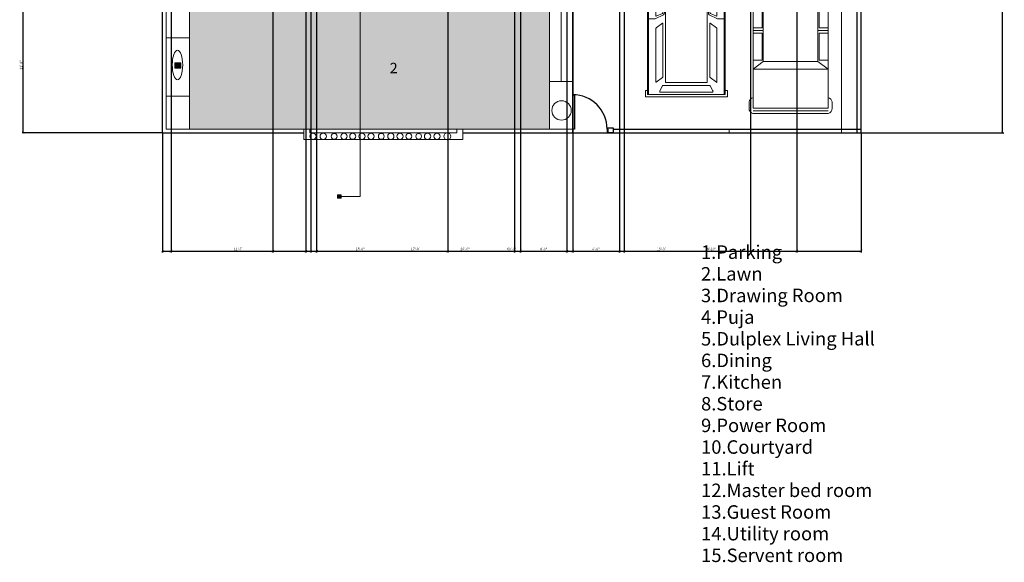
# Model space of a CAD drawing. Units: inches. Extents: x 3122 to 5933, y 1474 to 2995.
# Tile 3 of 12: x 4918 to 5933, y 1474 to 2032. Entities that reach past the tile are written whole.
import ezdxf

# ---------------------------------------------------------------- set-up
doc = ezdxf.new("R2010")
doc.units = ezdxf.units.IN
for name, color, linetype, lineweight in [('A-ANNO-DIMS', 2, 'Continuous', 18), ('A-ANNO-SYMB', 6, 'Continuous', 18), ('A-ANNO-TEXT', 7, 'Continuous', 18), ('A-AREA-IDEN', 7, 'Continuous', 20), ('A-DETL-PATT', 8, 'Continuous', 13), ('A-DOOR', 4, 'Continuous', 25), ('A-EQPM-VEHI', 8, 'Continuous', 13), ('C-PROP', 7, 'Continuous', 25), ('C-SITE', 8, 'Continuous', 18), ('L-PLNT', 3, 'Continuous', 18), ('L-PLNT-PATT', 94, 'Continuous', 13)]:
    doc.layers.add(name, color=color, linetype=linetype, lineweight=lineweight)
doc.styles.get("Standard").update_dxf_attribs({"font": 'arial.ttf'})
doc.dimstyles.new('ISO-25', dxfattribs={"dimtxt": 2.5, "dimasz": 2.5, "dimexe": 1.25, "dimexo": 0.625, "dimtad": 1, "dimdec": 0, "dimlunit": 3, "dimtxsty": 'Standard', "dimblk": 'ARCHTICK', "dimcen": 2.5, "dimadec": 0, "dimazin": 0, "dimtfac": 1, "dimtdec": 0, "dimtmove": 0, "dimatfit": 3, "dimfxl": 1, "dimarcsym": 0})

# ---------------------------------------------------------------- blocks, each defined once
blk = doc.blocks.new('*U24')
for p, q in [((5.4, 42.3), (12.1, 42.3)), ((189.7, 42.3), (183, 42.3)), ((0.1, -0.4), (0.1, 38.3)), ((2.8, -0.4), (2.8, 38.3)), ((5.4, 38.3), (16.1, 38.3)), ((5.4, -0.4), (5.4, 38.2)), ((16.1, 38.3), (180.3, 38.3)), ((61.5, -0.4), (61.5, 38.3)), ((61.5, 38.3), (77.5, 27.6)), ((64.2, 38.3), (76.2, 30.3)), ((76.2, 30.3), (76.2, 38.3)), ((78.9, 38.3), (78.9, 29)), ((106.9, 29), (106.9, 38.3)), ((109.6, 27.6), (109.6, 38.3)), ((112.3, 38.3), (112.3, 29)), ((140.3, 29), (140.3, 38.3)), ((141.6, 27.6), (149.6, 38.3)), ((149.6, -0.4), (149.6, 38.3)), ((189.7, 38.3), (179, 38.3)), ((189.7, -0.4), (189.7, 38.2)), ((192.4, -0.4), (192.4, 38.3)), ((195, -0.4), (195, 38.3)), ((77.5, 27.6), (141.6, 27.6)), ((77.5, -0.4), (77.5, 27.6)), ((78.9, 29), (106.9, 29)), ((112.3, 29), (140.3, 29)), ((141.6, -0.4), (141.6, 27.6)), ((5.4, 7.6), (61.5, 15.6)), ((0.1, -0.4), (0.1, -39.2)), ((2.8, -0.4), (2.8, -39.1)), ((5.4, -0.4), (5.4, -39.1)), ((5.4, -8.4), (61.5, -16.4)), ((61.5, -0.4), (61.5, -39.1)), ((77.5, -0.4), (77.5, -28.5)), ((141.6, -0.4), (141.6, -28.5)), ((149.6, -0.4), (149.6, -39.1)), ((189.7, -0.4), (189.7, -39.1)), ((192.4, -0.4), (192.4, -39.1)), ((195, -0.4), (195, -39.2)), ((61.5, -39.1), (77.5, -28.5)), ((77.5, -28.5), (141.6, -28.5)), ((78.9, -39.1), (78.9, -29.8)), ((78.9, -29.8), (106.9, -29.8)), ((106.9, -29.8), (106.9, -39.1)), ((109.6, -28.5), (109.6, -39.1)), ((112.3, -29.8), (140.3, -29.8)), ((112.3, -39.1), (112.3, -29.8)), ((140.3, -29.8), (140.3, -39.1)), ((141.6, -28.5), (149.6, -39.1)), ((5.4, -39.1), (16.1, -39.1)), ((16.1, -39.1), (180.3, -39.1)), ((64.2, -39.1), (76.2, -31.1)), ((76.2, -31.1), (76.2, -39.1)), ((189.7, -39.1), (179, -39.1)), ((5.4, -43.1), (12.1, -43.1)), ((189.7, -43.1), (183, -43.1))]:
    blk.add_line(p, q)
for centre, radius, start, end in [((5.1, 37.3), 5.06, 85.6455, 168.0943), ((11.5, 37.6), 4.72, 8.1301, 81.87), ((183.7, 37.6), 4.72, 98.13, 171.8699), ((190.1, 37.3), 5.06, 11.9057, 94.3545), ((5.1, -38.1), 5.06, 191.9057, 274.3545), ((11.5, -38.5), 4.72, 278.13, 351.8699), ((183.7, -38.5), 4.72, 188.1301, 261.87), ((190.1, -38.1), 5.06, 265.6455, 348.0943)]:
    blk.add_arc(centre, radius, start, end)
blk = doc.blocks.new('*U25')
for p, q in [((0, 0), (0, -100)), ((900, 0), (900, -100))]:
    blk.add_line(p, q)
blk.add_lwpolyline([(0, 0), (0, 900), (43.75, 900), (43.75, 0)], close=True)
blk.add_arc((0, 0), 900, 0, 90)
blk = doc.blocks.new('*U36')
for p, q in [((1.3, 38.9), (175.7, 38.9)), ((1.3, 28.1), (52.1, 28.1)), ((1.3, -28.1), (52.1, -28.1)), ((1.3, -38.9), (175.7, -38.9))]:
    blk.add_line(p, q)
for points in [[(5.6, 40), (5.6, 42.2), (0, 42.2), (0, -42.2), (5.6, -42.2), (5.6, -40), (1.3, -40), (1.3, 40)], [(171.7, 40), (175.7, 40), (175.7, -40), (171.7, -40), (171.7, -42.2), (178.1, -42.2), (178.1, 42.2), (171.7, 42.2)], [(1.3, 40), (175.7, 40), (175.7, -40), (1.3, -40)], [(71.5, 21.5), (163.4, 21.5), (163.4, -21.5), (71.5, -21.5)]]:
    blk.add_lwpolyline(points, close=True)
for points in [[(57.1, 40), (57.1, 32.4), (71.7, 22.8, 0.086577), (72.6, 22.7), (91.6, 22.7, 0.227875), (93.5, 23.6), (97.7, 32.1), (97.7, 40)], [(57.1, -40), (57.1, -32.4), (71.7, -22.8, -0.086577), (72.6, -22.7), (91.6, -22.7, -0.227875), (93.5, -23.6), (97.7, -32.1), (97.7, -40)]]:
    blk.add_lwpolyline(points, format="xyb")
for points in [[(62.1, 30.9), (72.1, 24.3, 0.146139), (72.7, 24.2), (91.4, 24.2, 0.29766), (92.3, 24.8), (95.1, 31.1, 0.541236), (94.9, 31.4), (62.2, 31.4, 0.744989)], [(102.2, 24.6), (107, 31, -0.236929), (107.8, 31.4), (162.9, 31.4, -0.621576), (163.1, 31), (158.2, 24.6, -0.233368), (157.4, 24.2), (102.4, 24.2, -0.616908)], [(55.5, 27.4), (68.6, 20.9, -0.284287), (69.1, 20), (69.1, -20, -0.284287), (68.6, -20.9), (55.5, -27.4, -0.557284), (54, -26.5), (54, 26.5, -0.557284)], [(171.9, 27.3), (166.8, 24.5, 0.271143), (166.3, 23.6), (166.3, -23.6, 0.271143), (166.8, -24.5), (171.9, -27.3, 0.573387), (173.4, -26.4), (173.4, 26.4, 0.573387)], [(62.1, -30.9), (72.1, -24.3, -0.146139), (72.7, -24.2), (91.4, -24.2, -0.29766), (92.3, -24.8), (95.1, -31.1, -0.541236), (94.9, -31.4), (62.2, -31.4, -0.744989)], [(102.2, -24.6), (107, -31, 0.236929), (107.8, -31.4), (162.9, -31.4, 0.621576), (163.1, -31), (158.2, -24.6, 0.233368), (157.4, -24.2), (102.4, -24.2, 0.616908)]]:
    blk.add_lwpolyline(points, format="xyb", close=True)
blk = doc.blocks.new('SECTION-LINE-END-MARK')
h = blk.add_hatch(color=256)
h.dxf.hatch_style = 1
h.paths.add_polyline_path([(3.7, 3.5), (0, 3.5), (0, 0), (3.7, 0)])
blk.add_lwpolyline([(0, 3.5), (3.7, 3.5), (3.7, 0), (0, 0)], close=True)
blk = doc.blocks.new('_ArchTick')
at = {"color": 0, "linetype": 'ByBlock', "const_width": 0.15}
blk.add_lwpolyline([(-0.5, -0.5), (0.5, 0.5)], dxfattribs=at)
blk = doc.blocks.new('*D92')
at = {"layer": 'A-ANNO-DIMS', "color": 0, "lineweight": -2, "transparency": 16777216}
for p, q in [((5065, 1915.3), (5065, 1792.9)), ((5785, 1915.3), (5785, 1792.9)), ((5065, 1794.2), (5785, 1794.2))]:
    blk.add_line(p, q, dxfattribs=at)
at = {"layer": 'Defpoints', "color": 0, "transparency": 16777216}
for p in [(5065, 1915.9), (5785, 1915.9), (5785, 1794.2)]:
    blk.add_point(p, dxfattribs=at)
at = {"layer": 'A-ANNO-DIMS', "color": 0, "lineweight": -2, "transparency": 16777216, "xscale": 2.5, "yscale": 2.5, "zscale": 2.5, "rotation": 180}
blk.add_blockref('_ArchTick', (5065, 1794.2), dxfattribs=at)
at = {"layer": 'A-ANNO-DIMS', "color": 0, "lineweight": -2, "transparency": 16777216, "xscale": 2.5, "yscale": 2.5, "zscale": 2.5}
blk.add_blockref('_ArchTick', (5785, 1794.2), dxfattribs=at)
at = {"layer": 'A-ANNO-DIMS', "color": 0, "transparency": 16777216, "insert": (5425, 1796.1), "char_height": 2.5, "attachment_point": 5}
blk.add_mtext('60\'-0"', dxfattribs=at)
blk = doc.blocks.new('*D93')
at = {"layer": 'A-ANNO-DIMS', "color": 0, "lineweight": -2, "transparency": 16777216}
for p, q in [((5785.6, 2875.9), (5932, 2875.9)), ((5930.7, 1915.9), (5930.7, 2875.9)), ((5785.6, 1915.9), (5932, 1915.9))]:
    blk.add_line(p, q, dxfattribs=at)
at = {"layer": 'Defpoints', "color": 0, "transparency": 16777216}
for p in [(5785, 2875.9), (5930.7, 2875.9), (5785, 1915.9)]:
    blk.add_point(p, dxfattribs=at)
at = {"layer": 'A-ANNO-DIMS', "color": 0, "lineweight": -2, "transparency": 16777216, "xscale": 2.5, "yscale": 2.5, "zscale": 2.5}
for p, rotation in [((5930.7, 2875.9), 90), ((5930.7, 1915.9), 270)]:
    blk.add_blockref('_ArchTick', p, dxfattribs=dict(at, rotation=rotation))
at = {"layer": 'A-ANNO-DIMS', "color": 0, "transparency": 16777216, "insert": (5928.8, 2395.9), "char_height": 2.5, "attachment_point": 5, "rotation": 90}
blk.add_mtext('80\'-0"', dxfattribs=at)
blk = doc.blocks.new('*D94')
at = {"layer": 'A-ANNO-DIMS', "color": 0, "lineweight": -2, "transparency": 16777216}
for p, q in [((5065, 1916.5), (5065, 2990.8)), ((5065, 2989.5), (5487.9, 2989.5)), ((5487.9, 1916.5), (5487.9, 2990.8))]:
    blk.add_line(p, q, dxfattribs=at)
at = {"layer": 'Defpoints', "color": 0, "transparency": 16777216}
for p in [(5487.9, 2989.5), (5065, 1915.9), (5487.9, 1915.9)]:
    blk.add_point(p, dxfattribs=at)
at = {"layer": 'A-ANNO-DIMS', "color": 0, "lineweight": -2, "transparency": 16777216, "xscale": 2.5, "yscale": 2.5, "zscale": 2.5, "rotation": 180}
blk.add_blockref('_ArchTick', (5065, 2989.5), dxfattribs=at)
at = {"layer": 'A-ANNO-DIMS', "color": 0, "lineweight": -2, "transparency": 16777216, "xscale": 2.5, "yscale": 2.5, "zscale": 2.5}
blk.add_blockref('_ArchTick', (5487.9, 2989.5), dxfattribs=at)
at = {"layer": 'A-ANNO-DIMS', "color": 0, "transparency": 16777216, "insert": (5276.4, 2991.4), "char_height": 2.5, "attachment_point": 5}
blk.add_mtext('35\'-3"', dxfattribs=at)
blk = doc.blocks.new('*D97')
at = {"layer": 'A-ANNO-DIMS', "color": 0, "lineweight": -2, "transparency": 16777216}
for p, q in [((5064.3, 2055.7), (4920.4, 2055.7)), ((4921.6, 1915.9), (4921.6, 2055.7)), ((5064.3, 1915.9), (4920.4, 1915.9))]:
    blk.add_line(p, q, dxfattribs=at)
at = {"layer": 'Defpoints', "color": 0, "transparency": 16777216}
for p in [(4921.6, 2055.7), (5065, 2055.7), (5065, 1915.9)]:
    blk.add_point(p, dxfattribs=at)
at = {"layer": 'A-ANNO-DIMS', "color": 0, "lineweight": -2, "transparency": 16777216, "xscale": 2.5, "yscale": 2.5, "zscale": 2.5}
for p, rotation in [((4921.6, 2055.7), 90), ((4921.6, 1915.9), 270)]:
    blk.add_blockref('_ArchTick', p, dxfattribs=dict(at, rotation=rotation))
at = {"layer": 'A-ANNO-DIMS', "color": 0, "transparency": 16777216, "insert": (4919.7, 1985.8), "char_height": 2.5, "attachment_point": 5, "rotation": 90}
blk.add_mtext('11\'-8"', dxfattribs=at)
blk = doc.blocks.new('*D102')
at = {"layer": 'A-ANNO-DIMS', "color": 0, "lineweight": -2, "transparency": 16777216}
for p, q in [((5074, 2064.1), (5074, 1792.9)), ((5213, 2064.1), (5213, 1792.9)), ((5074, 1794.2), (5213, 1794.2))]:
    blk.add_line(p, q, dxfattribs=at)
at = {"layer": 'Defpoints', "color": 0, "transparency": 16777216}
for p in [(5074, 2064.7), (5213, 2064.7), (5213, 1794.2)]:
    blk.add_point(p, dxfattribs=at)
at = {"layer": 'A-ANNO-DIMS', "color": 0, "lineweight": -2, "transparency": 16777216, "xscale": 2.5, "yscale": 2.5, "zscale": 2.5, "rotation": 180}
blk.add_blockref('_ArchTick', (5074, 1794.2), dxfattribs=at)
at = {"layer": 'A-ANNO-DIMS', "color": 0, "lineweight": -2, "transparency": 16777216, "xscale": 2.5, "yscale": 2.5, "zscale": 2.5}
blk.add_blockref('_ArchTick', (5213, 1794.2), dxfattribs=at)
at = {"layer": 'A-ANNO-DIMS', "color": 0, "transparency": 16777216, "insert": (5143.5, 1796.1), "char_height": 2.5, "attachment_point": 5}
blk.add_mtext('11\'-7"', dxfattribs=at)
blk = doc.blocks.new('*D103')
at = {"layer": 'A-ANNO-DIMS', "color": 0, "lineweight": -2, "transparency": 16777216}
for p, q in [((5224, 2112.1), (5224, 1792.9)), ((5427.9, 2112.1), (5427.9, 1792.9)), ((5224, 1794.2), (5427.9, 1794.2))]:
    blk.add_line(p, q, dxfattribs=at)
at = {"layer": 'Defpoints', "color": 0, "transparency": 16777216}
for p in [(5224, 2112.7), (5427.9, 2112.7), (5427.9, 1794.2)]:
    blk.add_point(p, dxfattribs=at)
at = {"layer": 'A-ANNO-DIMS', "color": 0, "lineweight": -2, "transparency": 16777216, "xscale": 2.5, "yscale": 2.5, "zscale": 2.5, "rotation": 180}
blk.add_blockref('_ArchTick', (5224, 1794.2), dxfattribs=at)
at = {"layer": 'A-ANNO-DIMS', "color": 0, "lineweight": -2, "transparency": 16777216, "xscale": 2.5, "yscale": 2.5, "zscale": 2.5}
blk.add_blockref('_ArchTick', (5427.9, 1794.2), dxfattribs=at)
at = {"layer": 'A-ANNO-DIMS', "color": 0, "transparency": 16777216, "insert": (5325.9, 1796.1), "char_height": 2.5, "attachment_point": 5}
blk.add_mtext('17\'-0"', dxfattribs=at)
blk = doc.blocks.new('*D105')
at = {"layer": 'A-ANNO-DIMS', "color": 0, "lineweight": -2, "transparency": 16777216}
for p, q in [((5433.9, 2249.8), (5433.9, 1792.9)), ((5481.9, 2249.8), (5481.9, 1792.9)), ((5433.9, 1794.2), (5481.9, 1794.2))]:
    blk.add_line(p, q, dxfattribs=at)
at = {"layer": 'Defpoints', "color": 0, "transparency": 16777216}
for p in [(5433.9, 2250.4), (5481.9, 2250.4), (5481.9, 1794.2)]:
    blk.add_point(p, dxfattribs=at)
at = {"layer": 'A-ANNO-DIMS', "color": 0, "lineweight": -2, "transparency": 16777216, "xscale": 2.5, "yscale": 2.5, "zscale": 2.5, "rotation": 180}
blk.add_blockref('_ArchTick', (5433.9, 1794.2), dxfattribs=at)
at = {"layer": 'A-ANNO-DIMS', "color": 0, "lineweight": -2, "transparency": 16777216, "xscale": 2.5, "yscale": 2.5, "zscale": 2.5}
blk.add_blockref('_ArchTick', (5481.9, 1794.2), dxfattribs=at)
at = {"layer": 'A-ANNO-DIMS', "color": 0, "transparency": 16777216, "insert": (5457.9, 1796.1), "char_height": 2.5, "attachment_point": 5}
blk.add_mtext('4\'-0"', dxfattribs=at)
blk = doc.blocks.new('*D106')
at = {"layer": 'A-ANNO-DIMS', "color": 0, "lineweight": -2, "transparency": 16777216}
for p, q in [((5540.9, 2249.9), (5540.9, 1792.9)), ((5718.7, 2249.9), (5718.7, 1792.9)), ((5540.9, 1794.2), (5718.7, 1794.2))]:
    blk.add_line(p, q, dxfattribs=at)
at = {"layer": 'Defpoints', "color": 0, "transparency": 16777216}
for p in [(5540.9, 2250.5), (5718.7, 2250.5), (5718.7, 1794.2)]:
    blk.add_point(p, dxfattribs=at)
at = {"layer": 'A-ANNO-DIMS', "color": 0, "lineweight": -2, "transparency": 16777216, "xscale": 2.5, "yscale": 2.5, "zscale": 2.5, "rotation": 180}
blk.add_blockref('_ArchTick', (5540.9, 1794.2), dxfattribs=at)
at = {"layer": 'A-ANNO-DIMS', "color": 0, "lineweight": -2, "transparency": 16777216, "xscale": 2.5, "yscale": 2.5, "zscale": 2.5}
blk.add_blockref('_ArchTick', (5718.7, 1794.2), dxfattribs=at)
at = {"layer": 'A-ANNO-DIMS', "color": 0, "transparency": 16777216, "insert": (5629.8, 1796.1), "char_height": 2.5, "attachment_point": 5}
blk.add_mtext('14\'-10"', dxfattribs=at)
blk = doc.blocks.new('*D108')
at = {"layer": 'A-ANNO-DIMS', "color": 0, "lineweight": -2, "transparency": 16777216}
for p, q in [((5179, 2643.1), (5179, 1792.9)), ((5359, 2643.1), (5359, 1792.9)), ((5179, 1794.2), (5359, 1794.2))]:
    blk.add_line(p, q, dxfattribs=at)
at = {"layer": 'Defpoints', "color": 0, "transparency": 16777216}
for p in [(5179, 2643.7), (5359, 2643.7), (5359, 1794.2)]:
    blk.add_point(p, dxfattribs=at)
at = {"layer": 'A-ANNO-DIMS', "color": 0, "lineweight": -2, "transparency": 16777216, "xscale": 2.5, "yscale": 2.5, "zscale": 2.5, "rotation": 180}
blk.add_blockref('_ArchTick', (5179, 1794.2), dxfattribs=at)
at = {"layer": 'A-ANNO-DIMS', "color": 0, "lineweight": -2, "transparency": 16777216, "xscale": 2.5, "yscale": 2.5, "zscale": 2.5}
blk.add_blockref('_ArchTick', (5359, 1794.2), dxfattribs=at)
at = {"layer": 'A-ANNO-DIMS', "color": 0, "transparency": 16777216, "insert": (5269, 1796.1), "char_height": 2.5, "attachment_point": 5}
blk.add_mtext('15\'-0"', dxfattribs=at)
blk = doc.blocks.new('*D110')
at = {"layer": 'A-ANNO-DIMS', "color": 0, "lineweight": -2, "transparency": 16777216}
for p, q in [((5487.9, 2643.1), (5487.9, 1792.9)), ((5671, 2643.1), (5671, 1792.9)), ((5487.9, 1794.2), (5671, 1794.2))]:
    blk.add_line(p, q, dxfattribs=at)
at = {"layer": 'Defpoints', "color": 0, "transparency": 16777216}
for p in [(5487.9, 2643.7), (5671, 2643.7), (5671, 1794.2)]:
    blk.add_point(p, dxfattribs=at)
at = {"layer": 'A-ANNO-DIMS', "color": 0, "lineweight": -2, "transparency": 16777216, "xscale": 2.5, "yscale": 2.5, "zscale": 2.5, "rotation": 180}
blk.add_blockref('_ArchTick', (5487.9, 1794.2), dxfattribs=at)
at = {"layer": 'A-ANNO-DIMS', "color": 0, "lineweight": -2, "transparency": 16777216, "xscale": 2.5, "yscale": 2.5, "zscale": 2.5}
blk.add_blockref('_ArchTick', (5671, 1794.2), dxfattribs=at)
at = {"layer": 'A-ANNO-DIMS', "color": 0, "transparency": 16777216, "insert": (5579.4, 1796.1), "char_height": 2.5, "attachment_point": 5}
blk.add_mtext('15\'-3"', dxfattribs=at)
blk = doc.blocks.new('*D115')
at = {"layer": 'A-ANNO-DIMS', "color": 0, "lineweight": -2, "transparency": 16777216}
for p, q in [((5218, 2532.1), (5218, 1792.9)), ((5535.9, 2532.1), (5535.9, 1792.9)), ((5218, 1794.2), (5535.9, 1794.2))]:
    blk.add_line(p, q, dxfattribs=at)
at = {"layer": 'Defpoints', "color": 0, "transparency": 16777216}
for p in [(5218, 2532.7), (5535.9, 2532.7), (5535.9, 1794.2)]:
    blk.add_point(p, dxfattribs=at)
at = {"layer": 'A-ANNO-DIMS', "color": 0, "lineweight": -2, "transparency": 16777216, "xscale": 2.5, "yscale": 2.5, "zscale": 2.5, "rotation": 180}
blk.add_blockref('_ArchTick', (5218, 1794.2), dxfattribs=at)
at = {"layer": 'A-ANNO-DIMS', "color": 0, "lineweight": -2, "transparency": 16777216, "xscale": 2.5, "yscale": 2.5, "zscale": 2.5}
blk.add_blockref('_ArchTick', (5535.9, 1794.2), dxfattribs=at)
at = {"layer": 'A-ANNO-DIMS', "color": 0, "transparency": 16777216, "insert": (5376.9, 1796.1), "char_height": 2.5, "attachment_point": 5}
blk.add_mtext('26\'-6"', dxfattribs=at)
blk = doc.blocks.new('*D117')
at = {"layer": 'A-ANNO-DIMS', "color": 0, "lineweight": -2, "transparency": 16777216}
for p, q in [((5488.5, 2244.4), (5932, 2244.4)), ((5930.7, 1915.9), (5930.7, 2244.4)), ((5488.5, 1915.9), (5932, 1915.9))]:
    blk.add_line(p, q, dxfattribs=at)
at = {"layer": 'Defpoints', "color": 0, "transparency": 16777216}
for p in [(5487.9, 2244.4), (5930.7, 2244.4), (5487.9, 1915.9)]:
    blk.add_point(p, dxfattribs=at)
at = {"layer": 'A-ANNO-DIMS', "color": 0, "lineweight": -2, "transparency": 16777216, "xscale": 2.5, "yscale": 2.5, "zscale": 2.5}
for p, rotation in [((5930.7, 2244.4), 90), ((5930.7, 1915.9), 270)]:
    blk.add_blockref('_ArchTick', p, dxfattribs=dict(at, rotation=rotation))
at = {"layer": 'A-ANNO-DIMS', "color": 0, "transparency": 16777216, "insert": (5928.8, 2080.1), "char_height": 2.5, "attachment_point": 5, "rotation": 90}
blk.add_mtext('27\'-4 1/2"', dxfattribs=at)
blk = doc.blocks.new('*D119')
at = {"layer": 'A-ANNO-DIMS', "color": 0, "lineweight": -2, "transparency": 16777216}
for p, q in [((5487.9, 2247.7), (5487.9, 1792.9)), ((5535.9, 2247.7), (5535.9, 1792.9)), ((5487.9, 1794.2), (5535.9, 1794.2))]:
    blk.add_line(p, q, dxfattribs=at)
at = {"layer": 'Defpoints', "color": 0, "transparency": 16777216}
for p in [(5487.9, 2248.3), (5535.9, 2248.3), (5535.9, 1794.2)]:
    blk.add_point(p, dxfattribs=at)
at = {"layer": 'A-ANNO-DIMS', "color": 0, "lineweight": -2, "transparency": 16777216, "xscale": 2.5, "yscale": 2.5, "zscale": 2.5, "rotation": 180}
blk.add_blockref('_ArchTick', (5487.9, 1794.2), dxfattribs=at)
at = {"layer": 'A-ANNO-DIMS', "color": 0, "lineweight": -2, "transparency": 16777216, "xscale": 2.5, "yscale": 2.5, "zscale": 2.5}
blk.add_blockref('_ArchTick', (5535.9, 1794.2), dxfattribs=at)
at = {"layer": 'A-ANNO-DIMS', "color": 0, "transparency": 16777216, "insert": (5511.9, 1796.1), "char_height": 2.5, "attachment_point": 5}
blk.add_mtext('4\'-0"', dxfattribs=at)

msp = doc.modelspace()

# ---------------------------------------------------------------- hatches: boundary and pattern name
at = {"layer": 'A-DETL-PATT'}
h = msp.add_hatch(color=256, dxfattribs=at)
h.dxf.hatch_style = 1
h.paths.add_polyline_path([(5084.21, 1988.18), (5078.02, 1988.18), (5078.02, 1982.65), (5084.21, 1982.65)])
at = {"layer": 'L-PLNT-PATT'}
h = msp.add_hatch(dxfattribs=at)
h.set_pattern_fill('GRASS', color=256, scale=0.1)
h.paths.add_polyline_path([(5463.87, 2047.66), (5427.87, 2047.66), (5217.96, 2047.66), (5217.96, 2055.71), (5092.96, 2055.71), (5092.96, 1919.9), (5463.87, 1919.9)])

# ---------------------------------------------------------------- linework, layer by layer
at = {"layer": 'A-ANNO-SYMB'}
for p, q in [((5268.96, 2933.31), (5268.96, 1850.37)), ((5268.96, 1850.37), (5249.31, 1850.37))]:
    msp.add_line(p, q, dxfattribs=at)
at = {"layer": 'C-PROP'}
for p, q in [((5064.96, 2875.9), (5064.96, 1915.9)), ((5784.96, 1915.9), (5784.96, 2875.9)), ((5780.96, 1915.9), (5780.96, 2245.15)), ((5487.87, 1919.9), (5487.87, 1915.9)), ((5523.87, 1919.9), (5523.87, 1915.9)), ((5529.36, 1919.9), (5784.96, 1919.9)), ((5064.96, 1915.9), (5210.91, 1915.9)), ((5374.55, 1915.9), (5487.87, 1915.9)), ((5523.87, 1915.9), (5784.96, 1915.9))]:
    msp.add_line(p, q, dxfattribs=at)
msp.add_lwpolyline([(5523.87, 1921), (5529.36, 1921), (5529.36, 1915.9), (5523.87, 1915.9)], close=True, dxfattribs=at)
at = {"layer": 'C-SITE'}
for p, q in [((5764.72, 1915.9), (5764.72, 2244.39)), ((5648.95, 1919.9), (5648.95, 1915.9))]:
    msp.add_line(p, q, dxfattribs=at)
at = {"layer": 'L-PLNT'}
for p, q in [((5068.96, 2055.71), (5068.96, 1919.9)), ((5092.96, 2055.71), (5092.96, 1919.9)), ((5463.87, 2047.66), (5463.87, 1919.9)), ((5475.87, 2047.66), (5475.87, 1968.97)), ((5487.87, 2047.66), (5487.87, 1919.9)), ((5068.96, 2013.88), (5092.96, 2013.88)), ((5463.87, 1968.97), (5487.87, 1968.97)), ((5068.96, 1953.88), (5092.96, 1953.88)), ((5068.96, 1919.9), (5487.87, 1919.9)), ((5210.91, 1909.25), (5210.91, 1919.9)), ((5216.91, 1915.9), (5216.91, 1919.9)), ((5368.55, 1919.9), (5368.55, 1915.9)), ((5374.55, 1919.9), (5374.55, 1909.25)), ((5374.55, 1909.25), (5210.91, 1909.25)), ((5216.91, 1915.9), (5368.55, 1915.9))]:
    msp.add_line(p, q, dxfattribs=at)
msp.add_lwpolyline([(5078.02, 1988.18), (5084.21, 1988.18), (5084.21, 1982.65), (5078.02, 1982.65)], close=True, dxfattribs=at)
for centre, radius in [((5476.3, 1939.03), 10), ((5220.26, 1912.39), 3.31), ((5230.75, 1912.39), 3.23), ((5242.07, 1912.39), 3.02), ((5252.2, 1912.39), 3.17), ((5261.19, 1912.39), 3.09), ((5270.73, 1912.39), 3.12), ((5279.95, 1912.39), 3.14), ((5290.58, 1912.39), 3.02), ((5300.43, 1912.39), 3.18), ((5309.92, 1912.39), 3.2), ((5318.98, 1912.39), 3.05), ((5329.09, 1912.39), 2.95), ((5338.25, 1912.39), 3.26), ((5348.09, 1912.39), 3.19), ((5358.63, 1912.39), 3.49)]:
    msp.add_circle(centre, radius, dxfattribs=at)
msp.add_ellipse((5080.6, 1985.83), major_axis=(0, -15.24), ratio=0.3551841, dxfattribs=at)

# ---------------------------------------------------------------- block references
at = {"layer": 'A-ANNO-SYMB'}
msp.add_blockref('SECTION-LINE-END-MARK', (5245.49, 1848.68), dxfattribs=at)
at = {"layer": 'A-DOOR', "xscale": 0.0393700787401575, "yscale": 0.0393700787401575, "zscale": 0.0393700787401575}
msp.add_blockref('*U25', (5487.87, 1919.83), dxfattribs=at)
at = {"layer": 'A-EQPM-VEHI', "rotation": 270}
for name, p in [('*U36', (5604.98, 2131.12)), ('*U24', (5712.74, 2131.01))]:
    msp.add_blockref(name, p, dxfattribs=at)

# ---------------------------------------------------------------- texts
at = {"layer": 'A-ANNO-TEXT'}
for s, height, p in [('1.Parking', 13.878, (5619.99, 1786.19)), ('2.Lawn', 13.878, (5620, 1763.9)), ('3.Drawing Room', 13.8775, (5620.01, 1741.61)), ('4.Puja', 13.878, (5620.02, 1719.32)), ('5.Dulplex Living Hall', 13.8775, (5620.04, 1697.02)), ('6.Dining', 13.878, (5620.05, 1674.73)), ('7.Kitchen', 13.878, (5620.06, 1652.44)), ('8.Store', 13.878, (5620.08, 1630.14)), ('9.Power Room', 13.8775, (5620.09, 1607.85)), ('10.Courtyard', 13.8775, (5620.1, 1585.56)), ('11.Lift', 13.878, (5620.12, 1563.26)), ('12.Master bed room', 13.8775, (5620.13, 1540.97)), ('13.Guest Room', 13.8775, (5620.14, 1518.68)), ('14.Utility room', 13.8775, (5620.15, 1496.39)), ('15.Servent room', 13.8775, (5620.17, 1474.09))]:
    msp.add_text(s, height=height, rotation=0.03333, dxfattribs=at).set_placement(p)
at = {"layer": 'A-AREA-IDEN'}
msp.add_text('2', height=10.72, rotation=0.03333, dxfattribs=at).set_placement((5299.35, 1977.32))

# ---------------------------------------------------------------- dimensions: what is measured, and where the dimension line sits
at = {"layer": 'A-ANNO-DIMS'}
for base, p1, p2, picture, middle in [((5487.87, 2989.5), (5064.96, 1915.9), (5487.87, 1915.9), '*D94', (5276.42, 2991.41)), ((5358.96, 1794.18), (5178.96, 2643.69), (5358.96, 2643.69), '*D108', (5268.96, 1796.08)), ((5670.96, 1794.18), (5487.87, 2643.69), (5670.96, 2643.69), '*D110', (5579.42, 1796.09)), ((5535.87, 1794.18), (5217.96, 2532.69), (5535.87, 2532.69), '*D115', (5376.92, 1796.08)), ((5481.87, 1794.18), (5433.87, 2250.39), (5481.87, 2250.39), '*D105', (5457.87, 1796.08)), ((5535.87, 1794.18), (5487.87, 2248.32), (5535.87, 2248.32), '*D119', (5511.87, 1796.08)), ((5718.65, 1794.18), (5540.87, 2250.49), (5718.65, 2250.49), '*D106', (5629.76, 1796.08)), ((5427.87, 1794.18), (5223.96, 2112.69), (5427.87, 2112.69), '*D103', (5325.92, 1796.08)), ((5212.96, 1794.18), (5073.96, 2064.71), (5212.96, 2064.71), '*D102', (5143.46, 1796.06)), ((5784.96, 1794.18), (5064.96, 1915.9), (5784.96, 1915.9), '*D92', (5424.96, 1796.08))]:
    dim = msp.add_linear_dim(base=base, p1=p1, p2=p2, dimstyle='ISO-25', override={"dimdec": 1, "dimlfac": 1, "dimrnd": 0, "dimzin": 1, "dimdsep": 46, "dimlunit": 4, "dimfrac": 2}, dxfattribs=at)
    dim.commit()
    dim.dimension.update_dxf_attribs({"geometry": picture, "text_midpoint": middle})
for base, p1, p2, picture, middle in [((5930.73, 2875.9), (5784.96, 1915.9), (5784.96, 2875.9), '*D93', (5928.83, 2395.9)), ((5930.73, 2244.39), (5487.87, 1915.9), (5487.87, 2244.39), '*D117', (5928.81, 2080.14)), ((4921.61, 2055.71), (5064.96, 1915.9), (5064.96, 2055.71), '*D97', (4919.71, 1985.8))]:
    dim = msp.add_linear_dim(base=base, p1=p1, p2=p2, angle=90, dimstyle='ISO-25', override={"dimdec": 1, "dimlfac": 1, "dimrnd": 0, "dimzin": 1, "dimdsep": 46, "dimlunit": 4, "dimfrac": 2}, dxfattribs=at)
    dim.commit()
    dim.dimension.update_dxf_attribs({"geometry": picture, "text_midpoint": middle})

doc.saveas('drawing.dxf')
